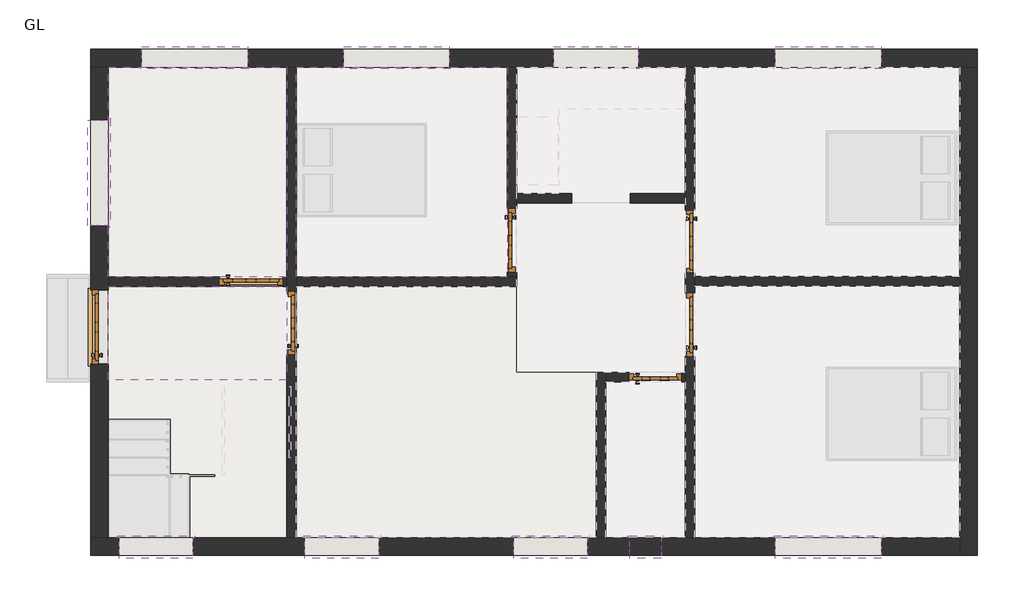
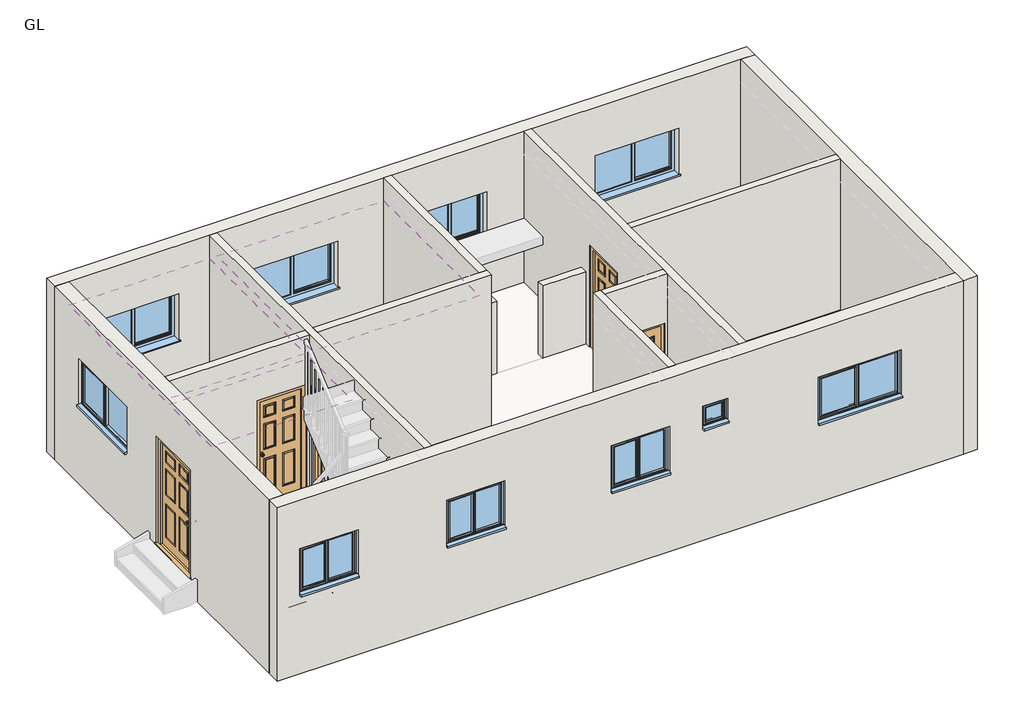
# One storey, part 1 of 2: 13 walls, 10 windows, 7 doors, 3 coverings, 3 slabs.
"""IFC4 building model written with IfcOpenShell, lengths in millimetres."""

from ifc_helpers import new_model, si_unit, frame, origin, origin_with_axes, place, context, project, spatial, polyline, outline, extrude, faceted_brep, transform, mapped, element, save
from components import doors_extsgl_11_2_5_c7418333, doors_extsgl_11_3_cb0934a6, doors_extsgl_11_3_1bca8958, doors_extsgl_11_3_5_304e37c5, windows_dbl_plain_3_5_9bb0dad6, windows_dbl_plain_4_0a19b8d2, windows_dbl_plain_5_b9c38b89, windows_sgl_plain_v_b14593de

model = new_model("IFC4")

# Units and contexts
model_context = context("Model", 3, world=origin())
ifc_project = project(units=[si_unit("LENGTHUNIT", "METRE", prefix="MILLI")], contexts=[model_context])

# Site, building, storey
site = spatial("IfcSite", under=ifc_project)
building = spatial("IfcBuilding", under=site)
storey = spatial("IfcBuildingStorey", under=building, Name="GL", Elevation=0.0)

# Coverings
placement = place(None, origin())
element("IfcCovering", 1, ObjectType="Plain", at=placement, inside=storey, context=model_context, shape_type="SweptSolid", body=[
    extrude(outline(polyline([(-4288.5477418, 6562.8522428), (-1717.6596772, 6562.8522428), (-1717.6596772, 3526.9173971), (-4288.5477418, 3526.9173971), (-4288.5477418, 6562.8522428)])), frame((0.0, 0.0, 2600.0), z_axis=(0.0, 0.0, 1.0), x_axis=(1.0, 0.0, 0.0)), (0.0, 0.0, 1.0), 57.0),
])
element("IfcCovering", 2, ObjectType="Plain", at=placement, inside=storey, context=model_context, shape_type="SweptSolid", body=[
    extrude(outline(polyline([(-4288.5477418, 3389.7573971), (-1717.6596772, 3389.7573971), (-1717.6596772, 2042.8185606), (-4288.5477418, 2042.8185606), (-4288.5477418, 3389.7573971)])), frame((0.0, 0.0, 2600.0), z_axis=(0.0, 0.0, 1.0), x_axis=(1.0, 0.0, 0.0)), (0.0, 0.0, 1.0), 57.0),
])
element("IfcCovering", 3, ObjectType="Plain", at=placement, inside=storey, context=model_context, shape_type="SweptSolid", body=[
    extrude(outline(polyline([(-1580.4996772, 6562.8522428), (1467.0922582, 6562.8522428), (1467.0922582, 3526.9173971), (-1580.4996772, 3526.9173971), (-1580.4996772, 6562.8522428)])), frame((0.0, 0.0, 2600.0), z_axis=(0.0, 0.0, 1.0), x_axis=(1.0, 0.0, 0.0)), (0.0, 0.0, 1.0), 57.0),
])

# Doors
doors_extsgl_11_2_5_shape = doors_extsgl_11_2_5_c7418333(model_context)
element("IfcDoor", 4, ObjectType="Doors_ExtSgl_11 : 2.5'", at=placement, inside=storey, context=model_context, shape_type="MappedRepresentation", body=[
    mapped(doors_extsgl_11_2_5_shape, transform((3602.1673421, 2084.8322428, 0.0), x_axis=(1.0, 0.0, 0.0), y_axis=(0.0, 1.0, 0.0), z_axis=(0.0, 0.0, 1.0))),
])
doors_extsgl_11_3_shape = doors_extsgl_11_3_cb0934a6(model_context)
element("IfcDoor", 5, ObjectType="Doors_ExtSgl_11 : 3'", at=placement, inside=storey, context=model_context, shape_type="MappedRepresentation", body=[
    mapped(doors_extsgl_11_3_shape, transform((-1649.0796772, 2864.6122428, 0.0), x_axis=(0.0, 1.0, 0.0), y_axis=(-1.0, 0.0, 0.0), z_axis=(0.0, 0.0, 1.0))),
])
element("IfcDoor", 6, ObjectType="Doors_ExtSgl_11 : 3'", at=placement, inside=storey, context=model_context, shape_type="MappedRepresentation", body=[
    mapped(doors_extsgl_11_3_shape, transform((1535.6722582, 4062.4009233, 0.0), x_axis=(0.0, -1.0, 0.0), y_axis=(1.0, 0.0, 0.0), z_axis=(0.0, 0.0, 1.0))),
])
element("IfcDoor", 7, ObjectType="Doors_ExtSgl_11 : 3'", at=placement, inside=storey, context=model_context, shape_type="MappedRepresentation", body=[
    mapped(doors_extsgl_11_3_shape, transform((4102.5473421, 2838.6460854, 0.0), x_axis=(0.0, 1.0, 0.0), y_axis=(-1.0, 0.0, 0.0), z_axis=(0.0, 0.0, 1.0))),
])
doors_extsgl_11_3_2_shape = doors_extsgl_11_3_1bca8958(model_context)
element("IfcDoor", 8, ObjectType="Doors_ExtSgl_11 : 3'", at=placement, inside=storey, context=model_context, shape_type="MappedRepresentation", body=[
    mapped(doors_extsgl_11_3_2_shape, transform((-2231.1477418, 3458.3373971, 0.0), x_axis=(1.0, 0.0, 0.0), y_axis=(0.0, 1.0, 0.0), z_axis=(0.0, 0.0, 1.0))),
])
element("IfcDoor", 9, ObjectType="Doors_ExtSgl_11 : 3'", at=placement, inside=storey, context=model_context, shape_type="MappedRepresentation", body=[
    mapped(doors_extsgl_11_3_2_shape, transform((4102.5473421, 4042.6060854, 0.0), x_axis=(0.0, -1.0, 0.0), y_axis=(1.0, 0.0, 0.0), z_axis=(0.0, 0.0, 1.0))),
])
doors_extsgl_11_3_5_shape = doors_extsgl_11_3_5_304e37c5(model_context)
element("IfcDoor", 10, ObjectType="Doors_ExtSgl_11 : 3.5'", at=placement, inside=storey, context=model_context, shape_type="MappedRepresentation", body=[
    mapped(doors_extsgl_11_3_5_shape, transform((-4418.0877418, 2805.5573971, 0.0), x_axis=(0.0, 1.0, 0.0), y_axis=(-1.0, 0.0, 0.0), z_axis=(0.0, 0.0, 1.0))),
])

# Slabs
element("IfcSlab", 11, ObjectType="DRAWING FLOOR", at=placement, inside=storey, context=model_context, shape_type="SweptSolid", body=[
    extrude(outline(polyline([(-1723.9477418, 6562.8522428), (-1723.9477418, 3503.7573971), (-4288.5477418, 3503.7573971), (-4288.5477418, 6562.8522428), (-1723.9477418, 6562.8522428)])), frame((0.0, 0.0, -24.9936), z_axis=(0.0, 0.0, 1.0), x_axis=(1.0, 0.0, 0.0)), (0.0, 0.0, 1.0), 149.9616),
])
element("IfcSlab", 12, ObjectType="LIVING AND DRAWING FLOOR", at=placement, inside=storey, context=model_context, shape_type="Brep", body=[
    faceted_brep([(2751.2673421, -234.1877572, -24.9936), (-1580.4996772, -234.1877572, -24.9936), (-1580.4996772, 3526.9173971, -24.9936), (1594.5003228, 3526.9173971, -24.9936), (1594.5003228, 2153.4122428, -24.9936), (1604.2522582, 2153.4122428, -24.9936), (2751.2673421, 2153.4122428, -24.9936), (-1580.4996772, -234.1877572, 124.968), (2751.2673421, -234.1877572, 124.968), (2751.2673421, 2153.4122428, 124.968), (1604.2522582, 2153.4122428, 124.968), (1594.5003228, 2153.4122428, 124.968), (1594.5003228, 3389.7573971, 124.968), (1594.5003228, 3526.9173971, 124.968), (-1580.4996772, 3526.9173971, 124.968), (-1580.4996772, 3389.7573971, 124.968), (1594.5003228, 3526.9173971, 0.0)], [[[0, 1, 2, 3, 4, 5, 6]], [[7, 8, 9, 10, 11, 12, 13, 14, 15]], [[1, 0, 8, 7]], [[2, 1, 7, 15, 14]], [[3, 2, 14, 13, 16]], [[4, 3, 16, 13, 12, 11]], [[4, 11, 10, 9, 6, 5]], [[0, 6, 9, 8]]]),
])
element("IfcSlab", 13, ObjectType="STAIR CASE FLOOR", at=placement, inside=storey, context=model_context, shape_type="Brep", body=[
    faceted_brep([(-1580.4996772, 3389.7573971, -24.9936), (-1580.4996772, -234.1877572, -24.9936), (-4288.5477418, -234.1877572, -24.9936), (-4288.5477418, 3389.7573971, -24.9936), (-1580.4996772, 3389.7573971, 124.968), (-4288.5477418, 3389.7573971, 124.968), (-4288.5477418, -234.1877572, 124.968), (-1580.4996772, -234.1877572, 124.968), (-4288.5477418, 3389.7573971, 0.0)], [[[0, 1, 2, 3]], [[4, 5, 6, 7]], [[1, 0, 4, 7]], [[2, 1, 7, 6]], [[3, 2, 6, 5, 8]], [[0, 3, 8, 5, 4]]]),
])

# Walls
element("IfcWall", 14, at=placement, inside=storey, context=model_context, shape_type="Brep", body=[
    faceted_brep([(-4547.6277418, 6562.8522428, -304.8), (-4288.5477418, 6562.8522428, -304.8), (7994.8922582, 6562.8522428, -304.8), (8253.9722582, 6562.8522428, -304.8), (8253.9722582, 6562.8522428, 3048.0), (7994.8922582, 6562.8522428, 3048.0), (4171.1273421, 6562.8522428, 3048.0), (4033.9673421, 6562.8522428, 3048.0), (1604.2522582, 6562.8522428, 3048.0), (1467.0922582, 6562.8522428, 3048.0), (-1580.4996772, 6562.8522428, 3048.0), (-1717.6596772, 6562.8522428, 3048.0), (-4288.5477418, 6562.8522428, 3048.0), (-4547.6277418, 6562.8522428, 3048.0), (-3805.9477418, 6562.8522428, 2110.0), (-2281.9477418, 6562.8522428, 2110.0), (-2281.9477418, 6562.8522428, 1200.0), (-3805.9477418, 6562.8522428, 1200.0), (-894.6996772, 6562.8522428, 2110.0), (629.3003228, 6562.8522428, 2110.0), (629.3003228, 6562.8522428, 1200.0), (-894.6996772, 6562.8522428, 1200.0), (2137.6522582, 6562.8522428, 2110.0), (3356.8522582, 6562.8522428, 2110.0), (3356.8522582, 6562.8522428, 1200.0), (2137.6522582, 6562.8522428, 1200.0), (5338.5757576, 6562.8522428, 2110.0), (6862.5757576, 6562.8522428, 2110.0), (6862.5757576, 6562.8522428, 1200.0), (5338.5757576, 6562.8522428, 1200.0), (-4547.6277418, 6821.9322428, -304.8), (-4547.6277418, 6821.9322428, 3048.0), (8253.9722582, 6821.9322428, 3048.0), (8253.9722582, 6821.9322428, -304.8), (-3805.9477418, 6821.9322428, 2110.0), (-3805.9477418, 6821.9322428, 1200.0), (-2281.9477418, 6821.9322428, 1200.0), (-2281.9477418, 6821.9322428, 2110.0), (-894.6996772, 6821.9322428, 2110.0), (-894.6996772, 6821.9322428, 1200.0), (629.3003228, 6821.9322428, 1200.0), (629.3003228, 6821.9322428, 2110.0), (2137.6522582, 6821.9322428, 2110.0), (2137.6522582, 6821.9322428, 1200.0), (3356.8522582, 6821.9322428, 1200.0), (3356.8522582, 6821.9322428, 2110.0), (5338.5757576, 6821.9322428, 2110.0), (5338.5757576, 6821.9322428, 1200.0), (6862.5757576, 6821.9322428, 1200.0), (6862.5757576, 6821.9322428, 2110.0)], [[[0, 1, 2, 3, 4, 5, 6, 7, 8, 9, 10, 11, 12, 13], [14, 15, 16, 17], [18, 19, 20, 21], [22, 23, 24, 25], [26, 27, 28, 29]], [[30, 31, 32, 33], [34, 35, 36, 37], [38, 39, 40, 41], [42, 43, 44, 45], [46, 47, 48, 49]], [[3, 2, 1, 0, 30, 33]], [[4, 3, 33, 32]], [[0, 13, 31, 30]], [[35, 34, 14, 17]], [[36, 35, 17, 16]], [[37, 36, 16, 15]], [[34, 37, 15, 14]], [[39, 38, 18, 21]], [[40, 39, 21, 20]], [[41, 40, 20, 19]], [[38, 41, 19, 18]], [[43, 42, 22, 25]], [[44, 43, 25, 24]], [[45, 44, 24, 23]], [[42, 45, 23, 22]], [[47, 46, 26, 29]], [[48, 47, 29, 28]], [[49, 48, 28, 27]], [[46, 49, 27, 26]], [[13, 12, 11, 10, 9, 8, 7, 6, 5, 4, 32, 31]]]),
])
element("IfcWall", 15, at=placement, inside=storey, context=model_context, shape_type="Brep", body=[
    faceted_brep([(7994.8922582, 6562.8522428, -304.8), (7994.8922582, -234.1877572, -304.8), (7994.8922582, -493.2677572, -304.8), (7994.8922582, -493.2677572, 3048.0), (7994.8922582, -234.1877572, 3048.0), (7994.8922582, 3397.4460854, 3048.0), (7994.8922582, 3534.6060854, 3048.0), (7994.8922582, 6562.8522428, 3048.0), (8253.9722582, 6562.8522428, -304.8), (8253.9722582, 6562.8522428, 3048.0), (8253.9722582, -493.2677572, 3048.0), (8253.9722582, -493.2677572, -304.8)], [[[0, 1, 2, 3, 4, 5, 6, 7]], [[8, 9, 10, 11]], [[2, 1, 0, 8, 11]], [[0, 7, 9, 8]], [[3, 2, 11, 10]], [[7, 6, 5, 4, 3, 10, 9]]]),
])
element("IfcWall", 16, at=placement, inside=storey, context=model_context, shape_type="Brep", body=[
    faceted_brep([(-4547.6277418, -493.2677572, -304.8), (7994.8922582, -493.2677572, -304.8), (7994.8922582, -493.2677572, 3048.0), (-4547.6277418, -493.2677572, 3048.0), (3689.7973421, -493.2677572, 2286.0), (3689.7973421, -493.2677572, 1828.8), (3232.5973421, -493.2677572, 1828.8), (3232.5973421, -493.2677572, 2286.0), (6862.5757576, -493.2677572, 2110.0), (6862.5757576, -493.2677572, 1200.0), (5338.5757576, -493.2677572, 1200.0), (5338.5757576, -493.2677572, 2110.0), (2624.2673421, -493.2677572, 2110.0), (2624.2673421, -493.2677572, 1200.0), (1557.4673421, -493.2677572, 1200.0), (1557.4673421, -493.2677572, 2110.0), (-386.6996772, -493.2677572, 2110.0), (-386.6996772, -493.2677572, 1200.0), (-1453.4996772, -493.2677572, 1200.0), (-1453.4996772, -493.2677572, 2110.0), (-3069.3477418, -493.2677572, 2110.0), (-3069.3477418, -493.2677572, 1200.0), (-4136.1477418, -493.2677572, 1200.0), (-4136.1477418, -493.2677572, 2110.0), (-4547.6277418, -234.1877572, -304.8), (-4547.6277418, -234.1877572, 3048.0), (-4288.5477418, -234.1877572, 3048.0), (-1717.6596772, -234.1877572, 3048.0), (-1580.4996772, -234.1877572, 3048.0), (2751.2673421, -234.1877572, 3048.0), (2888.4273421, -234.1877572, 3048.0), (4033.9673421, -234.1877572, 3048.0), (4171.1273421, -234.1877572, 3048.0), (7994.8922582, -234.1877572, 3048.0), (7994.8922582, -234.1877572, -304.8), (-4288.5477418, -234.1877572, -304.8), (3689.7973421, -234.1877572, 2286.0), (3232.5973421, -234.1877572, 2286.0), (3232.5973421, -234.1877572, 1828.8), (3689.7973421, -234.1877572, 1828.8), (6862.5757576, -234.1877572, 2110.0), (5338.5757576, -234.1877572, 2110.0), (5338.5757576, -234.1877572, 1200.0), (6862.5757576, -234.1877572, 1200.0), (2624.2673421, -234.1877572, 2110.0), (1557.4673421, -234.1877572, 2110.0), (1557.4673421, -234.1877572, 1200.0), (2624.2673421, -234.1877572, 1200.0), (-386.6996772, -234.1877572, 2110.0), (-1453.4996772, -234.1877572, 2110.0), (-1453.4996772, -234.1877572, 1200.0), (-386.6996772, -234.1877572, 1200.0), (-3069.3477418, -234.1877572, 2110.0), (-4136.1477418, -234.1877572, 2110.0), (-4136.1477418, -234.1877572, 1200.0), (-3069.3477418, -234.1877572, 1200.0)], [[[0, 1, 2, 3], [4, 5, 6, 7], [8, 9, 10, 11], [12, 13, 14, 15], [16, 17, 18, 19], [20, 21, 22, 23]], [[24, 25, 26, 27, 28, 29, 30, 31, 32, 33, 34, 35], [36, 37, 38, 39], [40, 41, 42, 43], [44, 45, 46, 47], [48, 49, 50, 51], [52, 53, 54, 55]], [[1, 0, 24, 35, 34]], [[2, 1, 34, 33]], [[0, 3, 25, 24]], [[5, 4, 36, 39]], [[6, 5, 39, 38]], [[7, 6, 38, 37]], [[4, 7, 37, 36]], [[9, 8, 40, 43]], [[10, 9, 43, 42]], [[11, 10, 42, 41]], [[8, 11, 41, 40]], [[13, 12, 44, 47]], [[14, 13, 47, 46]], [[15, 14, 46, 45]], [[12, 15, 45, 44]], [[17, 16, 48, 51]], [[18, 17, 51, 50]], [[19, 18, 50, 49]], [[16, 19, 49, 48]], [[21, 20, 52, 55]], [[22, 21, 55, 54]], [[23, 22, 54, 53]], [[20, 23, 53, 52]], [[3, 2, 33, 32, 31, 30, 29, 28, 27, 26, 25]]]),
])
element("IfcWall", 17, at=placement, inside=storey, context=model_context, shape_type="Brep", body=[
    faceted_brep([(-4288.5477418, -234.1877572, -304.8), (-4288.5477418, 6562.8522428, -304.8), (-4288.5477418, 6562.8522428, 3048.0), (-4288.5477418, 3526.9173971, 3048.0), (-4288.5477418, 3389.7573971, 3048.0), (-4288.5477418, -234.1877572, 3048.0), (-4288.5477418, 4274.1568236, 2110.0), (-4288.5477418, 5798.1568236, 2110.0), (-4288.5477418, 5798.1568236, 1200.0), (-4288.5477418, 4274.1568236, 1200.0), (-4288.5477418, 2272.1573971, 2110.0), (-4288.5477418, 3338.9573971, 2110.0), (-4288.5477418, 3338.9573971, 0.0), (-4288.5477418, 2272.1573971, 0.0), (-4547.6277418, -234.1877572, -304.8), (-4547.6277418, -234.1877572, 3048.0), (-4547.6277418, 6562.8522428, 3048.0), (-4547.6277418, 6562.8522428, -304.8), (-4547.6277418, 4274.1568236, 2110.0), (-4547.6277418, 4274.1568236, 1200.0), (-4547.6277418, 5798.1568236, 1200.0), (-4547.6277418, 5798.1568236, 2110.0), (-4547.6277418, 2272.1573971, 2110.0), (-4547.6277418, 2272.1573971, 0.0), (-4547.6277418, 3338.9573971, 0.0), (-4547.6277418, 3338.9573971, 2110.0)], [[[0, 1, 2, 3, 4, 5], [6, 7, 8, 9], [10, 11, 12, 13]], [[14, 15, 16, 17], [18, 19, 20, 21], [22, 23, 24, 25]], [[1, 0, 14, 17]], [[2, 1, 17, 16]], [[0, 5, 15, 14]], [[19, 18, 6, 9]], [[20, 19, 9, 8]], [[21, 20, 8, 7]], [[18, 21, 7, 6]], [[23, 22, 10, 13]], [[24, 23, 13, 12]], [[25, 24, 12, 11]], [[22, 25, 11, 10]], [[5, 4, 3, 2, 16, 15]]]),
])
element("IfcWall", 18, ObjectType="INNER WALL", at=placement, inside=storey, context=model_context, shape_type="Brep", body=[
    faceted_brep([(-1580.4996772, 3321.8122428, 2110.0), (-1580.4996772, 3321.8122428, 0.0), (-1580.4996772, 6562.8522428, 0.0), (-1580.4996772, 6562.8522428, 3048.0), (-1580.4996772, 3526.9173971, 3048.0), (-1580.4996772, 3389.7573971, 3048.0), (-1580.4996772, -234.1877572, 3048.0), (-1580.4996772, -234.1877572, 0.0), (-1580.4996772, 2407.4122428, 0.0), (-1580.4996772, 2407.4122428, 2110.0), (-1717.6596772, 6562.8522428, 0.0), (-1717.6596772, 3526.9173971, 0.0), (-1717.6596772, 3389.7573971, 0.0), (-1717.6596772, 3321.8122428, 0.0), (-1717.6596772, 3321.8122428, 2110.0), (-1717.6596772, 2407.4122428, 2110.0), (-1717.6596772, 2407.4122428, 0.0), (-1717.6596772, -234.1877572, 0.0), (-1717.6596772, -234.1877572, 3048.0), (-1717.6596772, 3389.7573971, 3048.0), (-1717.6596772, 3526.9173971, 3048.0), (-1717.6596772, 6562.8522428, 3048.0)], [[[0, 1, 2, 3, 4, 5, 6, 7, 8, 9]], [[10, 11, 12, 13, 14, 15, 16, 17, 18, 19, 20, 21]], [[8, 7, 17, 16]], [[2, 1, 13, 12, 11, 10]], [[3, 2, 10, 21]], [[7, 6, 18, 17]], [[16, 15, 9, 8]], [[14, 13, 1, 0]], [[15, 14, 0, 9]], [[6, 5, 4, 3, 21, 20, 19, 18]]]),
])
element("IfcWall", 19, ObjectType="INNER WALL", at=placement, inside=storey, context=model_context, shape_type="Brep", body=[
    faceted_brep([(1604.2522582, 3389.7573971, 0.0), (1604.2522582, 3389.7573971, 3048.0), (-1580.4996772, 3389.7573971, 3048.0), (-1580.4996772, 3389.7573971, 124.968), (1594.5003228, 3389.7573971, 124.968), (1594.5003228, 3389.7573971, 0.0), (1604.2522582, 3526.9173971, 3048.0), (1604.2522582, 3526.9173971, 0.0), (1594.5003228, 3526.9173971, 0.0), (1594.5003228, 3526.9173971, 124.968), (-1580.4996772, 3526.9173971, 124.968), (-1580.4996772, 3526.9173971, 3048.0), (1467.0922582, 3526.9173971, 3048.0)], [[[0, 1, 2, 3, 4, 5]], [[6, 7, 8, 9, 10, 11, 12]], [[7, 0, 5, 8]], [[2, 11, 10, 3]], [[1, 0, 7, 6]], [[9, 4, 3, 10]], [[4, 9, 8, 5]], [[1, 6, 12, 11, 2]]]),
    faceted_brep([(-4288.5477418, 3389.7573971, 3048.0), (-4288.5477418, 3389.7573971, 124.968), (-4288.5477418, 3389.7573971, 0.0), (-2688.3477418, 3389.7573971, 0.0), (-2688.3477418, 3389.7573971, 2110.0), (-1773.9477418, 3389.7573971, 2110.0), (-1773.9477418, 3389.7573971, 0.0), (-1717.6596772, 3389.7573971, 0.0), (-1717.6596772, 3389.7573971, 3048.0), (-4288.5477418, 3526.9173971, 0.0), (-4288.5477418, 3526.9173971, 3048.0), (-1717.6596772, 3526.9173971, 3048.0), (-1717.6596772, 3526.9173971, 0.0), (-1773.9477418, 3526.9173971, 0.0), (-1773.9477418, 3526.9173971, 2110.0), (-2688.3477418, 3526.9173971, 2110.0), (-2688.3477418, 3526.9173971, 0.0)], [[[0, 1, 2, 3, 4, 5, 6, 7, 8]], [[9, 10, 11, 12, 13, 14, 15, 16]], [[2, 9, 16, 3]], [[12, 7, 6, 13]], [[2, 1, 0, 10, 9]], [[8, 7, 12, 11]], [[16, 15, 4, 3]], [[14, 13, 6, 5]], [[15, 14, 5, 4]], [[10, 0, 8, 11]]]),
])
element("IfcWall", 20, ObjectType="INNER WALL", at=placement, inside=storey, context=model_context, shape_type="Brep", body=[
    faceted_brep([(1604.2522582, 3526.9173971, 0.0), (1604.2522582, 3605.2009233, 0.0), (1604.2522582, 3605.2009233, 2110.0), (1604.2522582, 4519.6009233, 2110.0), (1604.2522582, 4519.6009233, 0.0), (1604.2522582, 4597.8844495, 0.0), (1604.2522582, 4735.0444495, 0.0), (1604.2522582, 6562.8522428, 0.0), (1604.2522582, 6562.8522428, 3048.0), (1604.2522582, 3526.9173971, 3048.0), (1467.0922582, 3605.2009233, 2110.0), (1467.0922582, 3605.2009233, 0.0), (1467.0922582, 3526.9173971, 0.0), (1467.0922582, 3526.9173971, 3048.0), (1467.0922582, 6562.8522428, 3048.0), (1467.0922582, 6562.8522428, 0.0), (1467.0922582, 4519.6009233, 0.0), (1467.0922582, 4519.6009233, 2110.0), (1594.5003228, 3526.9173971, 0.0)], [[[0, 1, 2, 3, 4, 5, 6, 7, 8, 9]], [[10, 11, 12, 13, 14, 15, 16, 17]], [[16, 15, 7, 6, 5, 4]], [[12, 11, 1, 0, 18]], [[0, 9, 13, 12, 18]], [[8, 7, 15, 14]], [[4, 3, 17, 16]], [[2, 1, 11, 10]], [[3, 2, 10, 17]], [[9, 8, 14, 13]]]),
])
element("IfcWall", 21, ObjectType="INNER WALL", at=placement, inside=storey, context=model_context, shape_type="SweptSolid", body=[
    extrude(outline(polyline([(2399.2722582, 4597.8844495), (1604.2522582, 4597.8844495), (1604.2522582, 4735.0444495), (2399.2722582, 4735.0444495), (2399.2722582, 4597.8844495)])), origin_with_axes(), (0.0, 0.0, 1.0), 1524.0),
])
element("IfcWall", 22, ObjectType="INNER WALL", at=placement, inside=storey, context=model_context, shape_type="Brep", body=[
    faceted_brep([(4171.1273421, 3295.8460854, 0.0), (4171.1273421, 3397.4460854, 0.0), (4171.1273421, 3534.6060854, 0.0), (4171.1273421, 3585.4060854, 0.0), (4171.1273421, 3585.4060854, 2110.0), (4171.1273421, 4499.8060854, 2110.0), (4171.1273421, 4499.8060854, 0.0), (4171.1273421, 6562.8522428, 0.0), (4171.1273421, 6562.8522428, 3048.0), (4171.1273421, 3534.6060854, 3048.0), (4171.1273421, 3397.4460854, 3048.0), (4171.1273421, -234.1877572, 3048.0), (4171.1273421, -234.1877572, 0.0), (4171.1273421, 2381.4460854, 0.0), (4171.1273421, 2381.4460854, 2110.0), (4171.1273421, 3295.8460854, 2110.0), (4033.9673421, 3585.4060854, 2110.0), (4033.9673421, 3585.4060854, 0.0), (4033.9673421, 3295.8460854, 0.0), (4033.9673421, 3295.8460854, 2110.0), (4033.9673421, 2381.4460854, 2110.0), (4033.9673421, 2381.4460854, 0.0), (4033.9673421, 2153.4122428, 0.0), (4033.9673421, 2016.2522428, 0.0), (4033.9673421, -234.1877572, 0.0), (4033.9673421, -234.1877572, 3048.0), (4033.9673421, 2016.2522428, 3048.0), (4033.9673421, 2153.4122428, 3048.0), (4033.9673421, 6562.8522428, 3048.0), (4033.9673421, 6562.8522428, 0.0), (4033.9673421, 4499.8060854, 0.0), (4033.9673421, 4499.8060854, 2110.0)], [[[0, 1, 2, 3, 4, 5, 6, 7, 8, 9, 10, 11, 12, 13, 14, 15]], [[16, 17, 18, 19, 20, 21, 22, 23, 24, 25, 26, 27, 28, 29, 30, 31]], [[13, 12, 24, 23, 22, 21]], [[30, 29, 7, 6]], [[18, 17, 3, 2, 1, 0]], [[8, 7, 29, 28]], [[12, 11, 25, 24]], [[21, 20, 14, 13]], [[19, 18, 0, 15]], [[20, 19, 15, 14]], [[6, 5, 31, 30]], [[4, 3, 17, 16]], [[5, 4, 16, 31]], [[11, 10, 9, 8, 28, 27, 26, 25]]]),
])
element("IfcWall", 23, ObjectType="INNER WALL", at=placement, inside=storey, context=model_context, shape_type="Brep", body=[
    faceted_brep([(2888.4273421, -234.1877572, 0.0), (2888.4273421, 2016.2522428, 0.0), (2888.4273421, 2153.4122428, 0.0), (2888.4273421, 2153.4122428, 3048.0), (2888.4273421, 2016.2522428, 3048.0), (2888.4273421, -234.1877572, 3048.0), (2751.2673421, -234.1877572, 0.0), (2751.2673421, -234.1877572, 3048.0), (2751.2673421, 2153.4122428, 3048.0), (2751.2673421, 2153.4122428, 0.0)], [[[0, 1, 2, 3, 4, 5]], [[6, 7, 8, 9]], [[2, 1, 0, 6, 9]], [[0, 5, 7, 6]], [[3, 2, 9, 8]], [[5, 4, 3, 8, 7]]]),
])
element("IfcWall", 24, ObjectType="INNER WALL", at=placement, inside=storey, context=model_context, shape_type="SweptSolid", body=[
    extrude(outline(polyline([(2110.0, 3983.1673421), (0.0, 3983.1673421), (0.0, 4033.9673421), (3048.0, 4033.9673421), (3048.0, 2888.4273421), (0.0, 2888.4273421), (0.0, 3221.1673421), (2110.0, 3221.1673421), (2110.0, 3983.1673421)])), frame((0.0, 2016.2522428, 0.0), z_axis=(0.0, 1.0, 0.0), x_axis=(0.0, 0.0, 1.0)), (0.0, 0.0, 1.0), 137.16),
])
element("IfcWall", 25, ObjectType="INNER WALL", at=placement, inside=storey, context=model_context, shape_type="SweptSolid", body=[
    extrude(outline(polyline([(4171.1273421, 3534.6060854), (7994.8922582, 3534.6060854), (7994.8922582, 3397.4460854), (4171.1273421, 3397.4460854), (4171.1273421, 3534.6060854)])), origin_with_axes(), (0.0, 0.0, 1.0), 3048.0),
])
element("IfcWall", 26, ObjectType="INNER WALL", at=placement, inside=storey, context=model_context, shape_type="SweptSolid", body=[
    extrude(outline(polyline([(4029.9522582, 4597.8844495), (3242.5522582, 4597.8844495), (3242.5522582, 4735.0444495), (4029.9522582, 4735.0444495), (4029.9522582, 4597.8844495)])), origin_with_axes(), (0.0, 0.0, 1.0), 1524.0),
])

# Windows
windows_dbl_plain_3_5_shape = windows_dbl_plain_3_5_9bb0dad6(model_context)
element("IfcWindow", 27, ObjectType="Windows_Dbl_Plain : 3.5'", at=placement, inside=storey, context=model_context, shape_type="MappedRepresentation", body=[
    mapped(windows_dbl_plain_3_5_shape, transform((1805.8673421, -355.2711894, 0.0), x_axis=(-1.0, 0.0, 0.0), y_axis=(0.0, -1.0, 0.0), z_axis=(0.0, 0.0, 1.0))),
])
element("IfcWindow", 28, ObjectType="Windows_Dbl_Plain : 3.5'", at=placement, inside=storey, context=model_context, shape_type="MappedRepresentation", body=[
    mapped(windows_dbl_plain_3_5_shape, transform((-1205.0996772, -355.2711894, 0.0), x_axis=(-1.0, 0.0, 0.0), y_axis=(0.0, -1.0, 0.0), z_axis=(0.0, 0.0, 1.0))),
])
element("IfcWindow", 29, ObjectType="Windows_Dbl_Plain : 3.5'", at=placement, inside=storey, context=model_context, shape_type="MappedRepresentation", body=[
    mapped(windows_dbl_plain_3_5_shape, transform((-3887.7477418, -355.2711894, 0.0), x_axis=(-1.0, 0.0, 0.0), y_axis=(0.0, -1.0, 0.0), z_axis=(0.0, 0.0, 1.0))),
])
windows_dbl_plain_4_shape = windows_dbl_plain_4_0a19b8d2(model_context)
element("IfcWindow", 30, ObjectType="Windows_Dbl_Plain : 4'", at=placement, inside=storey, context=model_context, shape_type="MappedRepresentation", body=[
    mapped(windows_dbl_plain_4_shape, transform((3032.2522582, 6683.9356749, 0.0), x_axis=(1.0, 0.0, 0.0), y_axis=(0.0, 1.0, 0.0), z_axis=(0.0, 0.0, 1.0))),
])
windows_dbl_plain_5_shape = windows_dbl_plain_5_b9c38b89(model_context)
element("IfcWindow", 31, ObjectType="Windows_Dbl_Plain : 5'", at=placement, inside=storey, context=model_context, shape_type="MappedRepresentation", body=[
    mapped(windows_dbl_plain_5_shape, transform((-2758.9477418, 6683.9356749, 0.0), x_axis=(1.0, 0.0, 0.0), y_axis=(0.0, 1.0, 0.0), z_axis=(0.0, 0.0, 1.0))),
])
element("IfcWindow", 32, ObjectType="Windows_Dbl_Plain : 5'", at=placement, inside=storey, context=model_context, shape_type="MappedRepresentation", body=[
    mapped(windows_dbl_plain_5_shape, transform((152.3003228, 6683.9356749, 0.0), x_axis=(1.0, 0.0, 0.0), y_axis=(0.0, 1.0, 0.0), z_axis=(0.0, 0.0, 1.0))),
])
element("IfcWindow", 33, ObjectType="Windows_Dbl_Plain : 5'", at=placement, inside=storey, context=model_context, shape_type="MappedRepresentation", body=[
    mapped(windows_dbl_plain_5_shape, transform((6385.5757576, 6683.9356749, 0.0), x_axis=(1.0, 0.0, 0.0), y_axis=(0.0, 1.0, 0.0), z_axis=(0.0, 0.0, 1.0))),
])
element("IfcWindow", 34, ObjectType="Windows_Dbl_Plain : 5'", at=placement, inside=storey, context=model_context, shape_type="MappedRepresentation", body=[
    mapped(windows_dbl_plain_5_shape, transform((5815.5757576, -355.2711894, 0.0), x_axis=(-1.0, 0.0, 0.0), y_axis=(0.0, -1.0, 0.0), z_axis=(0.0, 0.0, 1.0))),
])
element("IfcWindow", 35, ObjectType="Windows_Dbl_Plain : 5'", at=placement, inside=storey, context=model_context, shape_type="MappedRepresentation", body=[
    mapped(windows_dbl_plain_5_shape, transform((-4409.631174, 5321.1568236, 0.0), x_axis=(0.0, 1.0, 0.0), y_axis=(-1.0, 0.0, 0.0), z_axis=(0.0, 0.0, 1.0))),
])
windows_sgl_plain_v_shape = windows_sgl_plain_v_b14593de(model_context)
element("IfcWindow", 36, ObjectType="Windows_Sgl_Plain : V", at=placement, inside=storey, context=model_context, shape_type="MappedRepresentation", body=[
    mapped(windows_sgl_plain_v_shape, transform((3461.1973421, -355.2711894, 176.0), x_axis=(-1.0, 0.0, 0.0), y_axis=(0.0, -1.0, 0.0), z_axis=(0.0, 0.0, 1.0))),
])

save(model, "model.ifc")

# Revit data of these elements
# Type "Plain"
#   Keynote = "K40"
#   built-in parameter 1002203 = 1 (stored number, unit not read)
#   built-in parameter 1002202 = 1 (stored number, unit not read)
#   Layers, outside or top first: 45 mm "Metal Stud Layer" (function 1); 12 mm "Gypsum Wall Board" (function 1)
# Type "Doors_ExtSgl_11 : 2.5'"
#   Type Mark = "50"
#   Type Comments = "External Single"
#   Operation = "SingleSwingRight"
#   Construction Type Id = "MDOOR"
#   Keynote = "L20"
#   Analytic Construction = "Metal"
#   Wrap Layers (Int) from Ext = 177.5 mm
#   Wrap Layers (Ext) from Ext = 102.5 mm
#   Thickness = 44 mm
#   Stile Top of Lock rail = 1000 mm
#   Stile Top of Frieze Rail = 1625 mm
#   Stile Top Rail = 150 mm
#   Stile Shutting = 125 mm
#   Stile Muntin Rail = 125 mm
#   Stile Lock Rail = 175 mm
#   Stile Intermediate/Frieze = 125 mm
#   Stile Hanging = 125 mm
#   Stile Bottom Rail = 175 mm
#   Rough Width = 762 mm
#   Rough Height = 2110 mm
#   O/A Frame Width = 64 mm
#   Heat Transfer Coefficient (U) = 3.7021 W/(m²·K)
#   Handle Z Distance = 1000 mm
#   Glazing Thickness = 24 mm
#   FrameWidth = 42 mm
#   FrameOffset - External = 25 mm
#   FrameDepth = 89 mm
#   Door Panel Width = 659 mm
#   Door Panel Thickness = 44 mm
#   Door Panel Height = 2000 mm
#   Cill Thickness = 54.5 mm
#   Handle X Distance = 75 mm
#   Height = 2110 mm
#   Structural Tolerance = 6.5 mm
#   Tolerance = 3 mm
#   Undercut = 4 mm
#   Width = 762 mm
#   Cill Projection = 30 mm
#   Cill Extension = 25 mm
#   Cavity Closer Width = 50 mm
#   Cavity Closer Offset from Ext = 102.5 mm
#   Cavity Closer Depth = 85 mm
#   Vis - Ironmongery = yes
#   Vis - Cavity Closers = yes
#   Define Thermal Properties by = 1
#   Function = 1
#   Material Door = Door - Panel
#   Material Frame = Door - Frame/Mullion
#   Material Ironmongery = Door - Handle
#   Visual Light Transmittance = 0
#   Solar Heat Gain Coefficient = 0
#   Wall Closure = (empty or 0)
# Type "Doors_ExtSgl_11 : 3'"
#   Type Mark = "49"
#   Type Comments = "External Single"
#   Operation = "SingleSwingRight"
#   Construction Type Id = "MDOOR"
#   Keynote = "L20"
#   Analytic Construction = "Metal"
#   Wrap Layers (Int) from Ext = 177.5 mm
#   Wrap Layers (Ext) from Ext = 102.5 mm
#   Thickness = 44 mm
#   Stile Top of Lock rail = 1000 mm
#   Stile Top of Frieze Rail = 1625 mm
#   Stile Top Rail = 150 mm
#   Stile Shutting = 125 mm
#   Stile Muntin Rail = 125 mm
#   Stile Lock Rail = 175 mm
#   Stile Intermediate/Frieze = 125 mm
#   Stile Hanging = 125 mm
#   Stile Bottom Rail = 175 mm
#   Rough Width = 914.4 mm
#   Rough Height = 2110 mm
#   O/A Frame Width = 64 mm
#   Heat Transfer Coefficient (U) = 3.7021 W/(m²·K)
#   Handle Z Distance = 1000 mm
#   Glazing Thickness = 24 mm
#   FrameWidth = 42 mm
#   FrameOffset - External = 25 mm
#   FrameDepth = 89 mm
#   Door Panel Width = 811.4 mm
#   Door Panel Thickness = 44 mm
#   Door Panel Height = 2000 mm
#   Cill Thickness = 54.5 mm
#   Handle X Distance = 75 mm
#   Height = 2110 mm
#   Structural Tolerance = 6.5 mm
#   Tolerance = 3 mm
#   Undercut = 4 mm
#   Width = 914.4 mm
#   Cill Projection = 30 mm
#   Cill Extension = 25 mm
#   Cavity Closer Width = 50 mm
#   Cavity Closer Offset from Ext = 102.5 mm
#   Cavity Closer Depth = 85 mm
#   Vis - Ironmongery = yes
#   Vis - Cavity Closers = yes
#   Define Thermal Properties by = 1
#   Function = 1
#   Material Door = Door - Panel
#   Material Frame = Door - Frame/Mullion
#   Material Ironmongery = Door - Handle
#   Visual Light Transmittance = 0
#   Solar Heat Gain Coefficient = 0
#   Wall Closure = (empty or 0)
# Type "Doors_ExtSgl_11 : 3.5'"
#   Type Mark = "48"
#   Type Comments = "External Single"
#   Operation = "SingleSwingRight"
#   Construction Type Id = "MDOOR"
#   Keynote = "L20"
#   Analytic Construction = "Metal"
#   Wrap Layers (Int) from Ext = 177.5 mm
#   Wrap Layers (Ext) from Ext = 102.5 mm
#   Thickness = 44 mm
#   Stile Top of Lock rail = 1000 mm
#   Stile Top of Frieze Rail = 1625 mm
#   Stile Top Rail = 150 mm
#   Stile Shutting = 125 mm
#   Stile Muntin Rail = 125 mm
#   Stile Lock Rail = 175 mm
#   Stile Intermediate/Frieze = 125 mm
#   Stile Hanging = 125 mm
#   Stile Bottom Rail = 175 mm
#   Rough Width = 1066.8 mm
#   Rough Height = 2110 mm
#   O/A Frame Width = 64 mm
#   Heat Transfer Coefficient (U) = 3.7021 W/(m²·K)
#   Handle Z Distance = 1000 mm
#   Glazing Thickness = 24 mm
#   FrameWidth = 42 mm
#   FrameOffset - External = 25 mm
#   FrameDepth = 89 mm
#   Door Panel Width = 963.8 mm
#   Door Panel Thickness = 44 mm
#   Door Panel Height = 2000 mm
#   Cill Thickness = 54.5 mm
#   Handle X Distance = 75 mm
#   Height = 2110 mm
#   Structural Tolerance = 6.5 mm
#   Tolerance = 3 mm
#   Undercut = 4 mm
#   Width = 1066.8 mm
#   Cill Projection = 30 mm
#   Cill Extension = 25 mm
#   Cavity Closer Width = 50 mm
#   Cavity Closer Offset from Ext = 102.5 mm
#   Cavity Closer Depth = 85 mm
#   Vis - Ironmongery = yes
#   Vis - Cavity Closers = yes
#   Define Thermal Properties by = 1
#   Function = 1
#   Material Door = Door - Panel
#   Material Frame = Door - Frame/Mullion
#   Material Ironmongery = Door - Handle
#   Visual Light Transmittance = 0
#   Solar Heat Gain Coefficient = 0
#   Wall Closure = (empty or 0)
# Type "DRAWING FLOOR"
#   Function = 0
#   Layers, outside or top first: 21.946 mm "Wood Sheathing, Chipboard" (function 5); 128.016 mm "Structure, Timber Joist/Rafter Layer" (function 1)
# Type "LIVING AND DRAWING FLOOR"
#   Function = 0
#   Layers, outside or top first: 21.946 mm "Wood Sheathing, Chipboard" (function 5); 128.016 mm "Structure, Timber Joist/Rafter Layer" (function 1)
# Type "STAIR CASE FLOOR"
#   Function = 0
#   Layers, outside or top first: 21.946 mm "Wood Sheathing, Chipboard" (function 5); 128.016 mm "Structure, Timber Joist/Rafter Layer" (function 1)
# Type
#   Keynote = "F10"
#   Layers, outside or top first: 259.08 mm "Brick, Common" (function 1)
# Type "INNER WALL"
#   Keynote = "F10"
#   Layers, outside or top first: 137.16 mm "Brick, Common" (function 1)
# Type "Windows_Dbl_Plain : 3.5'"
#   Type Mark = "64"
#   Operation = "DoublePanelVertical"
#   Construction Type Id = "GSP4R"
#   Manufacturer = "Revit"
#   Keynote = "L10"
#   Analytic Construction = "1/8 in Pilkington single glazing"
#   Wrap Layers (Ext) from Ext = 102.5 mm
#   Wrap Layers (Int) from Ext = 177.5 mm
#   Window Board Projection = 25 mm
#   Window Board Extension = 25 mm
#   Visual Light Transmittance = 0.9
#   Solar Heat Gain Coefficient = 0.78
#   Rough Width = 1066.8 mm
#   Rough Height = 910 mm
#   Height = 910 mm
#   Width = 1066.8 mm
#   Heat Transfer Coefficient (U) = 3.6886 W/(m²·K)
#   Glazing Thickness = 24 mm
#   FrameOffset - External = 50 mm
#   Frame Depth = 65 mm
#   Default Head Height = 2110 mm
#   Cill Depth = 87.5 mm
#   Cavity Closer Width = 50 mm
#   Cavity Closer Offset from Ext = 102.5 mm
#   Cavity Closer Depth = 85 mm
#   Vis - Cavity Closers = yes
#   Define Thermal Properties by = 1
#   Material Trim = Window Frame
#   Material Glass = Glass
#   Material Frame = Window Frame
#   Wall Closure = (empty or 0)
# Type "Windows_Dbl_Plain : 4'"
#   Type Mark = "63"
#   Operation = "DoublePanelVertical"
#   Construction Type Id = "GSP4R"
#   Manufacturer = "Revit"
#   Keynote = "L10"
#   Analytic Construction = "1/8 in Pilkington single glazing"
#   Wrap Layers (Ext) from Ext = 102.5 mm
#   Wrap Layers (Int) from Ext = 177.5 mm
#   Window Board Projection = 25 mm
#   Window Board Extension = 25 mm
#   Visual Light Transmittance = 0.9
#   Solar Heat Gain Coefficient = 0.78
#   Rough Width = 1219.2 mm
#   Rough Height = 910 mm
#   Height = 910 mm
#   Width = 1219.2 mm
#   Heat Transfer Coefficient (U) = 3.6886 W/(m²·K)
#   Glazing Thickness = 24 mm
#   FrameOffset - External = 50 mm
#   Frame Depth = 65 mm
#   Default Head Height = 2110 mm
#   Cill Depth = 87.5 mm
#   Cavity Closer Width = 50 mm
#   Cavity Closer Offset from Ext = 102.5 mm
#   Cavity Closer Depth = 85 mm
#   Vis - Cavity Closers = yes
#   Define Thermal Properties by = 1
#   Material Trim = Window Frame
#   Material Glass = Glass
#   Material Frame = Window Frame
#   Wall Closure = (empty or 0)
# Type "Windows_Dbl_Plain : 5'"
#   Type Mark = "62"
#   Operation = "DoublePanelVertical"
#   Construction Type Id = "GSP4R"
#   Manufacturer = "Revit"
#   Keynote = "L10"
#   Analytic Construction = "1/8 in Pilkington single glazing"
#   Wrap Layers (Ext) from Ext = 102.5 mm
#   Wrap Layers (Int) from Ext = 177.5 mm
#   Window Board Projection = 25 mm
#   Window Board Extension = 25 mm
#   Visual Light Transmittance = 0.9
#   Solar Heat Gain Coefficient = 0.78
#   Rough Width = 1524 mm
#   Rough Height = 910 mm
#   Height = 910 mm
#   Width = 1524 mm
#   Heat Transfer Coefficient (U) = 3.6886 W/(m²·K)
#   Glazing Thickness = 24 mm
#   FrameOffset - External = 50 mm
#   Frame Depth = 65 mm
#   Default Head Height = 2110 mm
#   Cill Depth = 87.5 mm
#   Cavity Closer Width = 50 mm
#   Cavity Closer Offset from Ext = 102.5 mm
#   Cavity Closer Depth = 85 mm
#   Vis - Cavity Closers = yes
#   Define Thermal Properties by = 1
#   Material Trim = Window Frame
#   Material Glass = Glass
#   Material Frame = Window Frame
#   Wall Closure = (empty or 0)
# Type "Windows_Sgl_Plain : V"
#   Type Mark = "66"
#   Operation = "SinglePanel"
#   Construction Type Id = "SGL"
#   Manufacturer = "Revit"
#   Keynote = "L10"
#   Analytic Construction = "Large single-glazed windows"
#   Wrap Layers (Ext) from Ext = 102.5 mm
#   Wrap Layers (Int) from Ext = 177.5 mm
#   Window Board Projection = 25 mm
#   Window Board Extension = 25 mm
#   Visual Light Transmittance = 0.9
#   Solar Heat Gain Coefficient = 0.86
#   Rough Width = 457.2 mm
#   Rough Height = 457.2 mm
#   Height = 457.2 mm
#   Width = 457.2 mm
#   Heat Transfer Coefficient (U) = 5.5617 W/(m²·K)
#   Glazing Thickness = 24 mm
#   FrameOffset - External = 50 mm
#   Frame Depth = 65 mm
#   Default Head Height = 2110 mm
#   Cill Depth = 87.5 mm
#   Cavity Closer Width = 50 mm
#   Cavity Closer Offset from Ext = 102.5 mm
#   Cavity Closer Depth = 85 mm
#   Vis - Cavity Closers = yes
#   Define Thermal Properties by = 1
#   Material Trim = Window Frame
#   Material Glass = Glass
#   Material Frame = Window Frame
#   Wall Closure = (empty or 0)
# Elements 1, 2, 3 (IfcCovering, "Plain")
#   Height Offset From Level = 2600 mm
#   Phase Created = New Construction
#   Materials on its faces: "Gypsum Wall Board", "Metal Stud Layer"
# Element 4 (IfcDoor, "Doors_ExtSgl_11 : 2.5'")
#   Phase Created = New Construction
#   Materials on its faces: "Door - Panel", "Door - Handle", "Door - Frame/Mullion"
# Elements 5, 6, 7, 8, 9 (IfcDoor, "Doors_ExtSgl_11 : 3'")
#   Phase Created = New Construction
#   Materials on its faces: "Door - Panel", "Door - Handle", "Door - Frame/Mullion"
# Element 10 (IfcDoor, "Doors_ExtSgl_11 : 3.5'")
#   Phase Created = New Construction
#   Materials on its faces: "Door - Panel", "Door - Handle", "Door - Frame/Mullion"
# Element 11 (IfcSlab, "DRAWING FLOOR")
#   Height Offset From Level = 124.968 mm
#   Phase Created = New Construction
#   Materials on its faces: "Structure, Timber Joist/Rafter Layer", "Wood Sheathing, Chipboard"
# Element 12 (IfcSlab, "LIVING AND DRAWING FLOOR")
#   built-in parameter 1001955 = -1.5708 (stored number, unit not read)
#   Height Offset From Level = 124.968 mm
#   Phase Created = New Construction
#   Materials on its faces: "Structure, Timber Joist/Rafter Layer", "Wood Sheathing, Chipboard"
# Element 13 (IfcSlab, "STAIR CASE FLOOR")
#   Height Offset From Level = 124.968 mm
#   Phase Created = New Construction
#   Materials on its faces: "Structure, Timber Joist/Rafter Layer", "Wood Sheathing, Chipboard"
# Elements 14, 15, 16, 17 (IfcWall)
#   built-in parameter 1001111 = -304.8 mm
#   Top Offset = 0 mm
#   Base Offset = -304.8 mm
#   wall height = 3352.8 mm
#   Phase Created = New Construction
#   Base Constraint = GL
#   Top Constraint = TL
#   Materials on its faces: "Brick, Common"
# Elements 18, 19, 20, 22, 23, 24, 25 (IfcWall, "INNER WALL")
#   Top Offset = 0 mm
#   Base Offset = 0 mm
#   wall height = 3048 mm
#   Phase Created = New Construction
#   Base Constraint = GL
#   Top Constraint = TL
#   Materials on its faces: "Brick, Common"
# Elements 21, 26 (IfcWall, "INNER WALL")
#   Top Offset = -1524 mm
#   Base Offset = 0 mm
#   wall height = 1524 mm
#   Phase Created = New Construction
#   Base Constraint = GL
#   Top Constraint = TL
#   Materials on its faces: "Brick, Common"
# Element 27 (IfcWindow, "Windows_Dbl_Plain : 3.5'")
#   Mark = "7"
#   Phase Created = New Construction
#   Materials on its faces: "Window Frame", "Glass"
# Element 28 (IfcWindow, "Windows_Dbl_Plain : 3.5'")
#   Mark = "8"
#   Phase Created = New Construction
#   Materials on its faces: "Window Frame", "Glass"
# Element 29 (IfcWindow, "Windows_Dbl_Plain : 3.5'")
#   Mark = "9"
#   Phase Created = New Construction
#   Materials on its faces: "Window Frame", "Glass"
# Element 30 (IfcWindow, "Windows_Dbl_Plain : 4'")
#   Mark = "4"
#   Phase Created = New Construction
#   Materials on its faces: "Window Frame", "Glass"
# Element 31 (IfcWindow, "Windows_Dbl_Plain : 5'")
#   Mark = "2"
#   Phase Created = New Construction
#   Materials on its faces: "Window Frame", "Glass"
# Element 32 (IfcWindow, "Windows_Dbl_Plain : 5'")
#   Mark = "3"
#   Phase Created = New Construction
#   Materials on its faces: "Window Frame", "Glass"
# Element 33 (IfcWindow, "Windows_Dbl_Plain : 5'")
#   Mark = "5"
#   Phase Created = New Construction
#   Materials on its faces: "Window Frame", "Glass"
# Element 34 (IfcWindow, "Windows_Dbl_Plain : 5'")
#   Mark = "6"
#   Phase Created = New Construction
#   Materials on its faces: "Window Frame", "Glass"
# Element 35 (IfcWindow, "Windows_Dbl_Plain : 5'")
#   Mark = "10"
#   Phase Created = New Construction
#   Materials on its faces: "Window Frame", "Glass"
# Element 36 (IfcWindow, "Windows_Sgl_Plain : V")
#   Mark = "1"
#   Phase Created = New Construction
#   Materials on its faces: "Window Frame", "Glass"
# Materials
#   "Metal Stud Layer": class "Metal", colour RGB 127 127 127, transparency 0, Description = "Light gauge steel framing, thermal air layer", Cost = 0
#   "Gypsum Wall Board": class "Generic", colour RGB 249 249 249, transparency 0, Description = "Gypsum Wall Board", Cost = 0
#   "Door - Panel": class "Wood", colour RGB 210 159 95, transparency 0, Keynote = "L20", Cost = 0
#   "Door - Frame/Mullion": class "Wood", colour RGB 212 179 113, transparency 0, Keynote = "L20", Cost = 0
#   "Door - Handle": colour RGB 0 0 0, transparency 0, Keynote = "P21", Cost = 0
#   "Wood Sheathing, Chipboard": class "Wood", colour RGB 127 127 127, transparency 0, Description = "Particleboard sheathing", Cost = 0
#   "Structure, Timber Joist/Rafter Layer": class "Wood", colour RGB 127 127 127, transparency 0, Description = "Timber framing, thermal airspace", Cost = 0
#   "Brick, Common": class "Masonry", colour RGB 170 100 105, transparency 0, Description = "Common brick", Cost = 0
#   "Window Frame": colour RGB 249 249 249, transparency 0, Keynote = "L10", Cost = 0
#   "Glass": class "Glass", colour RGB 0 128 192, transparency 0.9, Description = "Soda Lime Glass", Cost = 0
